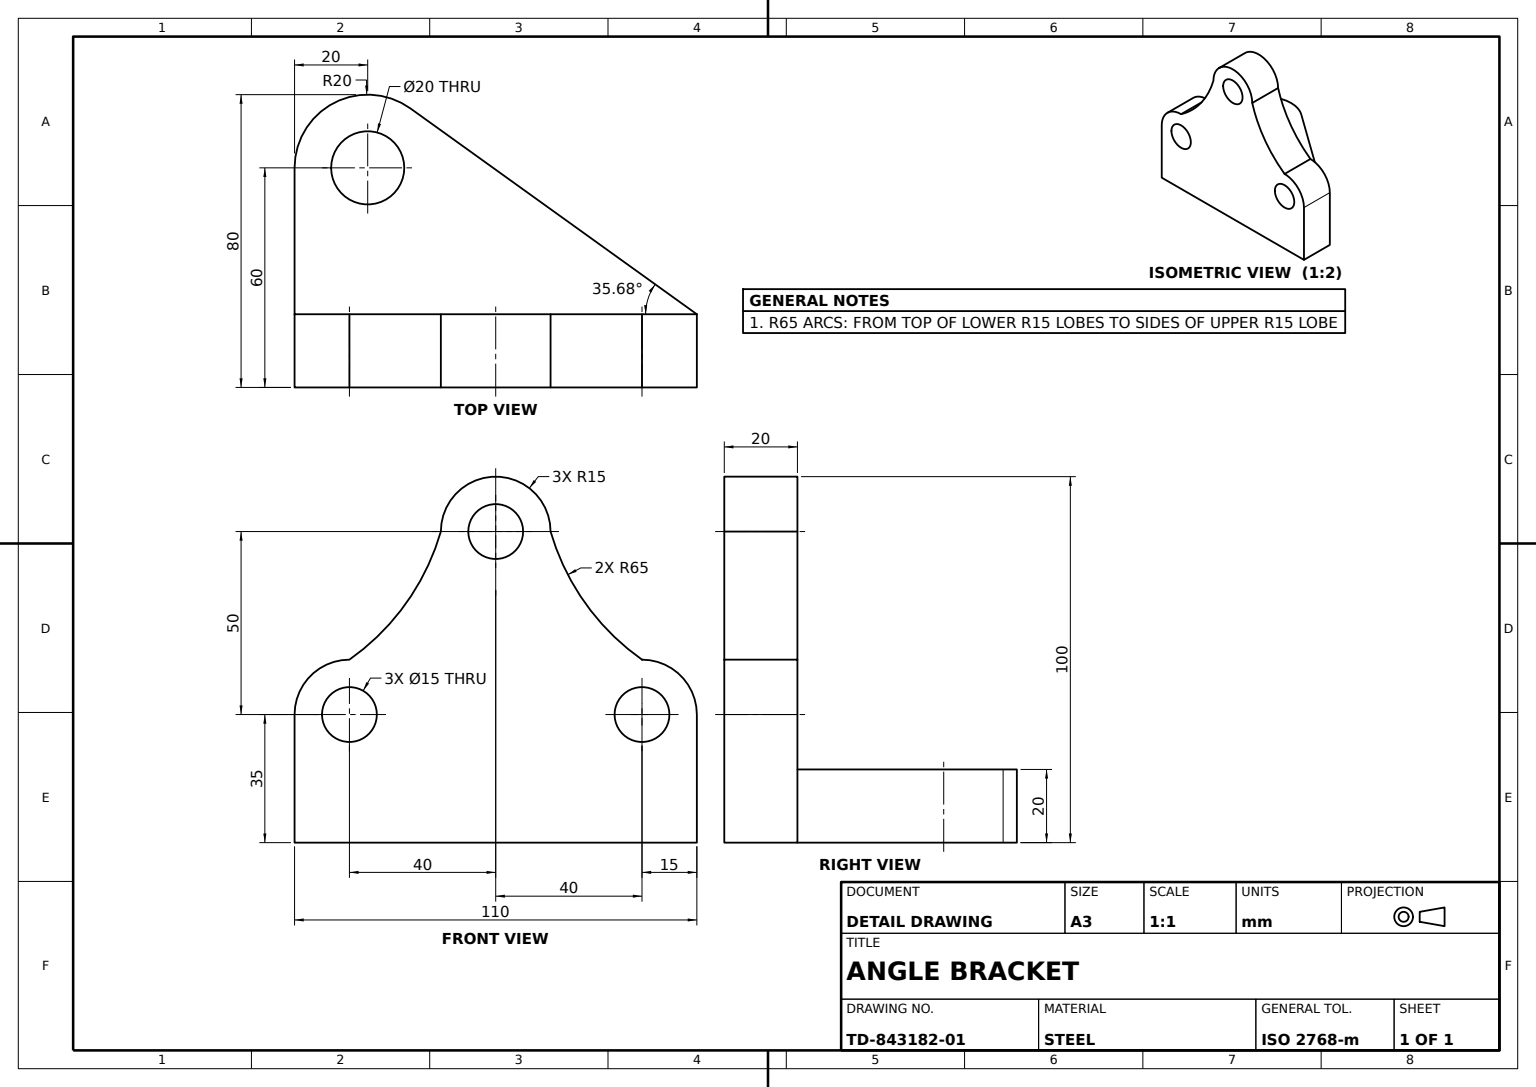
SolidWorks part; units mm, degrees
material "Plain Carbon Steel"
ref_plane "Front Plane" through (0, 0, 0) normal (0, 0, 1) x (1, 0, 0)
ref_plane "Top Plane" through (0, 0, 0) normal (0, 1, 0) x (1, 0, 0)
ref_plane "Right Plane" through (0, 0, 0) normal (1, 0, 0) x (0, 0, -1)
sketch "Bracket Profile Sketch" plane through (0, 0, 0) normal (1, 0, 0) x (0, 0, -1)
  line L2 (55, 0) -> (55, -15)
  line L3 (55, -15) -> (-55.0015, -15)
  line L4 (-55.0015, -15) -> (-55, 0)
  arc A0 (55, 0) -> (40, 15) centre (40, 0) ccw
  arc A1 (-40, 15) -> (-55, 0) centre (-40, 0) ccw
  arc A2 (15, 50) -> (-15, 50) centre (0, 50) ccw
  circle A3 centre (0, 50) radius 7.5
  circle A4 centre (40, 0) radius 7.5
  circle A5 centre (-40, 0) radius 7.5
  arc A6 (15, 50) -> (40, 15) centre (77.4138, 68.1527) ccw
  arc A7 (-15, 50) -> (-40, 15) centre (-77.4138, 68.1527) cw
  dimension "D1" = 15
  dimension "D2" = 15
  dimension "D3" = 15
  dimension "D4" = 15
  dimension "D5" = 15
  dimension "D6" = 15
  dimension "D7" = 40
  dimension "D10" = 65
  dimension "D8" = 40
  dimension "D9" = 50
  dimension "D11" = 15
  dimension "D12" = 110.0015
extrude "Bracket Profile Boss" add sketch "Bracket Profile Sketch" along normal blind 20
ref_plane "Base Block Plane" through (0, -15, 0) normal (0, -1, 0) x (-1, 0, 0)
sketch "Base Block Sketch" plane through (0, -15, 0) normal (0, -1, 0) x (-1, 0, 0)
  line L0 (-20, 55) -> (-20, -55.0015)
  line L1 (-20, -55.0015) -> (0, -55.0015)
  line L2 (40, -55.0015) -> (0, -55.0015)
  line L3 (-20, 55) -> (0, 55)
  line L4 (0, 55) -> (56.246, -23.3368)
  arc A0 (40, -55.0015) -> (56.246, -23.3368) centre (40, -35.0015) ccw
  circle A1 centre (40, -35.0015) radius 10
  dimension "D1" = 40
  dimension "D2" = 20
  dimension "D3" = 20
  dimension "D4" = 55
  dimension "D5" = 110.0015
  dimension "D6" = 40
  dimension "D7" = 96.4379
extrude "Base Block Boss" add sketch "Base Block Sketch" along normal blind 20
